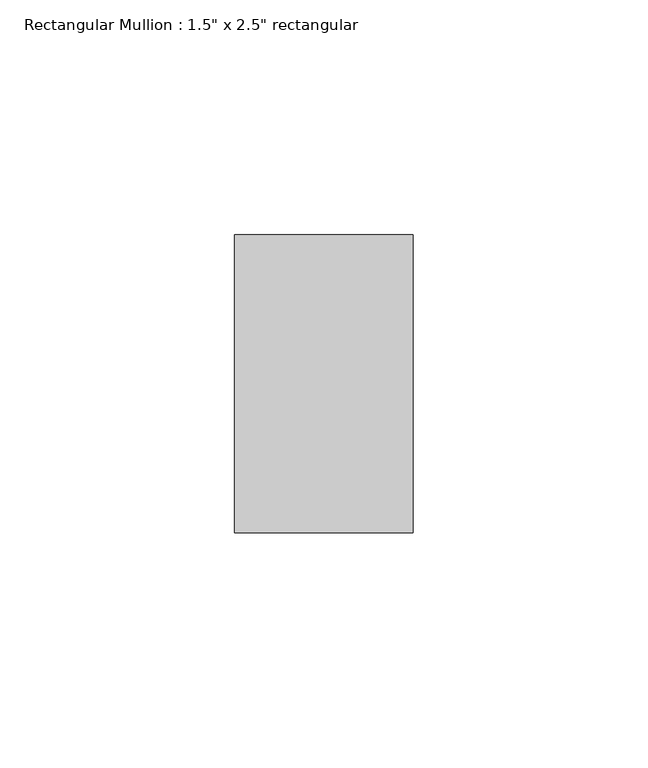
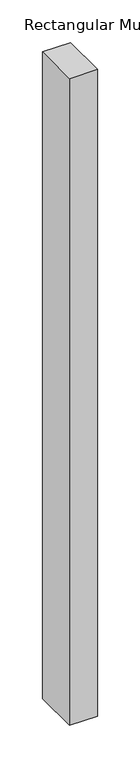
"""IFC4 building model written with IfcOpenShell, lengths in millimetres: member geometry."""

from ifc_helpers import new_model, si_unit, frame, origin, place, context, project, spatial, polyline, outline, extrude, source, transform, mapped, element, save


def member_51048147(model_context):
    return source(origin(), model_context, "Body", "SweptSolid", [
        extrude(outline(polyline([(19.05, 31.75), (19.05, -31.75), (-19.05, -31.75), (-19.05, 31.75), (19.05, 31.75)])), frame((0.0, 0.0, -927.1000003), z_axis=(0.0, 0.0, 1.0), x_axis=(1.0, 0.0, 0.0)), (0.0, 0.0, 1.0), 927.1000003),
    ])


if __name__ == "__main__":
    model = new_model("IFC4")
    model_context = context("Model", 3, world=origin())
    ifc_project = project(units=[si_unit("LENGTHUNIT", "METRE", prefix="MILLI")], contexts=[model_context])
    site = spatial("IfcSite", under=ifc_project)
    building = spatial("IfcBuilding", under=site)
    placement = place(None, origin())
    member_shape = member_51048147(model_context)
    element("IfcMember", 1, ObjectType="Rectangular Mullion : 1.5\" x 2.5\" rectangular", at=placement, inside=building, context=model_context, shape_type="MappedRepresentation", body=[
        mapped(member_shape, transform((0.0, 0.0, 0.0), x_axis=(1.0, 0.0, 0.0), y_axis=(0.0, 1.0, 0.0), z_axis=(0.0, 0.0, 1.0))),
    ])
    save(model, "model.ifc")

# Revit data of these elements
# Type "Rectangular Mullion : 1.5\" x 2.5\" rectangular"
#   built-in parameter 1007304 = 0.208333 (stored number, unit not read)
#   built-in parameter 1007301 = 0.0625 (stored number, unit not read)
#   built-in parameter 1007300 = 0.0625 (stored number, unit not read)
# Element 1 (IfcMember, "Rectangular Mullion : 1.5\" x 2.5\" rectangular")
#   Materials on its faces: "Aluminum"
# Materials
#   "Aluminum": class "Metal", colour RGB 247 247 247, transparency 0, Description = "Aluminum 6061", Cost = 0
